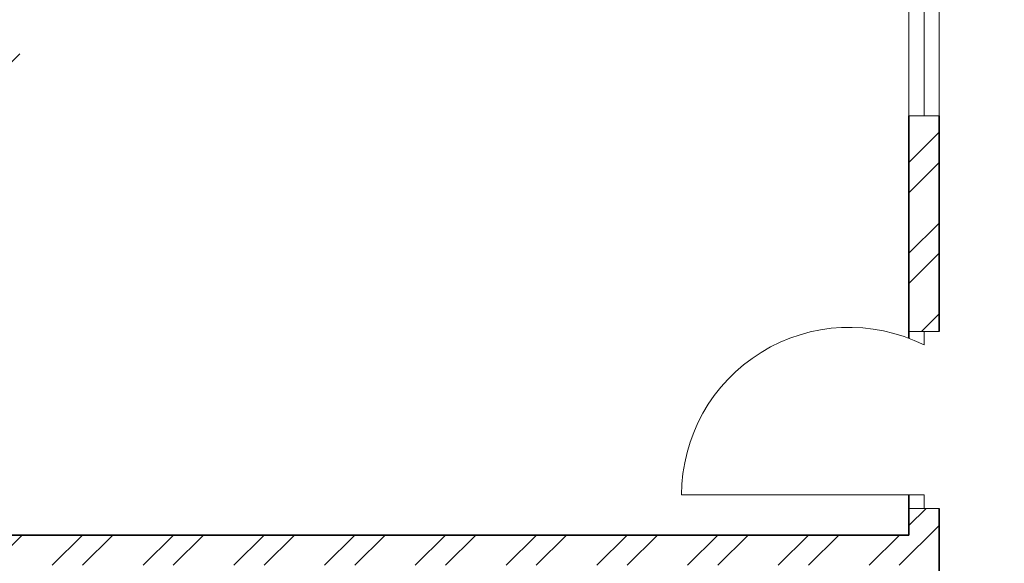
# Model space of a CAD drawing. Units: inches. Extents: x 1885 to 2748, y 783 to 2421.
# Tile 50 of 117: x 2311 to 2457, y 1683 to 1764. Entities that reach past the tile are written whole.
import ezdxf

# ---------------------------------------------------------------- set-up
doc = ezdxf.new("R2010")
doc.units = ezdxf.units.IN
for name, color, linetype, lineweight in [('A-DOOR', 31, 'Continuous', 18), ('A-GLAZ', 181, 'Continuous', 18), ('A-WALL', 7, 'Continuous', 35)]:
    doc.layers.add(name, color=color, linetype=linetype, lineweight=lineweight)
doc.layers.add('A-WALL-PATT', color=85, linetype='Continuous', lineweight=13, true_color=0x58ba48)

# ---------------------------------------------------------------- blocks, each defined once
blk = doc.blocks.new('WIN-60')
for p, q in [((0, 60), (4.5, 60)), ((0, 60), (0, 0)), ((4.5, 60), (2.25, 60)), ((2.25, 60), (2.25, 0)), ((4.5, 0), (4.5, 60)), ((2.25, 0), (0, 0)), ((0, 0), (4.5, 0))]:
    blk.add_line(p, q)

msp = doc.modelspace()

# ---------------------------------------------------------------- hatches: boundary and pattern name
at = {"layer": 'A-WALL-PATT'}
h = msp.add_hatch(dxfattribs=at)
h.set_pattern_fill('ANSI32', color=256)
h.paths.add_polyline_path([(2007.77, 2318.01), (1980.77, 2318.01), (1980.77, 2281.22), (1985.27, 2281.22), (1985.27, 2313.51), (2007.77, 2313.51), (2007.77, 2315.76)])
h.paths.add_polyline_path([(2094.32, 2318.01), (2067.77, 2318.01), (2067.77, 2313.51), (2094.32, 2313.51), (2094.32, 2315.76)])
h.paths.add_polyline_path([(2131.37, 2315.76), (2131.37, 2318.01), (2131.19, 2318.01), (2112.61, 2318.01), (2112.61, 2313.51), (2117.27, 2313.51), (2117.27, 2255.2), (2121.77, 2255.2), (2121.77, 2313.51), (2131.37, 2313.51)])
h.paths.add_polyline_path([(2190.51, 2318.01), (2155.37, 2318.01), (2155.37, 2313.51), (2169.77, 2313.51), (2169.77, 2229.51), (2121.77, 2229.51), (2121.77, 2233.45), (2119.52, 2233.45), (2117.27, 2233.45), (2117.27, 2201.1), (2121.77, 2201.1), (2121.77, 2225.01), (2169.77, 2225.01), (2169.77, 2165.01), (2306.27, 2165.01), (2306.27, 2066.01), (2310.77, 2066.01), (2344.27, 2066.01), (2486.27, 2066.01), (2486.27, 1886.01), (2483.02, 1886.01), (2483.02, 1881.51), (2486.27, 1881.51), (2486.27, 1880.68), (2490.77, 1880.68), (2490.77, 2070.51), (2344.27, 2070.51), (2310.77, 2070.51), (2310.77, 2165.01), (2310.77, 2173.64), (2308.52, 2173.64), (2306.27, 2173.64), (2306.27, 2169.51), (2174.27, 2169.51), (2174.27, 2313.51), (2190.51, 2313.51), (2190.51, 2315.76)])
h.paths.add_polyline_path([(1985.27, 2221.22), (1980.77, 2221.22), (1980.77, 2165.01), (1992.77, 2165.01), (1992.77, 2141.93), (1997.27, 2141.93), (1997.27, 2165.01), (2117.27, 2165.01), (2117.27, 2163.13), (2121.77, 2163.13), (2121.77, 2172.73), (2119.52, 2172.73), (2117.27, 2172.73), (2117.27, 2169.51), (1985.27, 2169.51)])
h.paths.add_polyline_path([(1997.27, 2105.93), (1992.77, 2105.93), (1992.77, 2070.51), (2016.77, 2070.51), (2016.77, 2059.12), (2019.02, 2059.12), (2021.27, 2059.12), (2021.27, 2070.51), (2117.27, 2070.51), (2117.27, 2022.51), (2114.42, 2022.51), (2114.42, 2018.01), (2123.63, 2018.01), (2123.63, 2020.26), (2123.63, 2022.51), (2121.77, 2022.51), (2121.77, 2142.59), (2119.52, 2142.59), (2117.27, 2142.59), (2117.27, 2075.01), (1997.27, 2075.01)])
h.paths.add_polyline_path([(2092.03, 2020.26), (2092.03, 2022.51), (2021.27, 2022.51), (2021.27, 2035.12), (2016.77, 2035.12), (2016.77, 2018.01), (2016.77, 1978.78), (2021.27, 1978.78), (2021.27, 2018.01), (2092.03, 2018.01)])
h.paths.add_polyline_path([(2260.94, 2022.51), (2153.1, 2022.51), (2153.1, 2020.26), (2153.1, 2018.01), (2155.27, 2018.01), (2155.27, 1886.01), (2107.63, 1886.01), (2107.63, 1881.51), (2182.91, 1881.51), (2182.91, 1883.76), (2182.91, 1886.01), (2159.77, 1886.01), (2159.77, 2018.01), (2260.94, 2018.01), (2260.94, 2020.26)])
h.paths.add_polyline_path([(2047.63, 1883.76), (2047.63, 1886.01), (2021.27, 1886.01), (2021.27, 1918.78), (2019.02, 1918.78), (2016.77, 1918.78), (2016.77, 1881.51), (2047.63, 1881.51)])
h.paths.add_polyline_path([(2306.36, 1883.76), (2306.36, 1886.01), (2296.27, 1886.01), (2296.27, 1982.01), (2316.54, 1982.01), (2316.54, 1984.26), (2316.54, 1986.51), (2296.27, 1986.51), (2296.27, 2022.51), (2289.28, 2022.51), (2289.28, 2018.01), (2291.77, 2018.01), (2291.77, 1886.01), (2242.91, 1886.01), (2242.91, 1881.51), (2306.36, 1881.51)], flags=17)
h.paths.add_polyline_path([(1985.27, 1843.01), (2021.6, 1843.01), (2021.53, 1845.44), (2021.48, 1847.51), (1980.77, 1847.51), (1980.77, 1809.45), (1985.27, 1809.45)])
h.paths.add_polyline_path([(2131.48, 1845.26), (2131.48, 1847.51), (2081.53, 1847.51), (2081.53, 1843.01), (2117.27, 1843.01), (2117.27, 1784.15), (2119.52, 1784.15), (2121.77, 1784.15), (2121.77, 1843.01), (2131.48, 1843.01)])
h.paths.add_polyline_path([(2203.89, 1847.51), (2155.48, 1847.51), (2155.48, 1843.01), (2169.77, 1843.01), (2169.77, 1759.01), (2121.77, 1759.01), (2121.77, 1761.46), (2117.27, 1761.46), (2117.27, 1730.43), (2121.77, 1730.43), (2121.77, 1754.51), (2177.42, 1754.51), (2177.42, 1756.76), (2177.42, 1759.01), (2174.27, 1759.01), (2174.27, 1843.01), (2203.89, 1843.01)])
h.paths.add_polyline_path([(2335.55, 1845.26), (2335.55, 1847.51), (2239.89, 1847.51), (2239.89, 1843.01), (2306.27, 1843.01), (2306.27, 1759.01), (2199.49, 1759.01), (2199.49, 1754.51), (2310.77, 1754.51), (2310.77, 1843.01), (2335.55, 1843.01)])
h.paths.add_polyline_path([(2348.77, 2022.51), (2344.27, 2022.51), (2344.27, 1986.51), (2341.68, 1986.51), (2341.68, 1982.01), (2344.27, 1982.01), (2344.27, 1886.01), (2330.36, 1886.01), (2330.36, 1881.51), (2361.63, 1881.51), (2361.63, 1883.76), (2361.63, 1886.01), (2348.77, 1886.01)], flags=17)
h.paths.add_polyline_path([(2283.25, 2315.76), (2283.25, 2318.01), (2238.51, 2318.01), (2238.51, 2313.51), (2283.25, 2313.51)], flags=17)
h.paths.add_polyline_path([(2363.27, 2348.01), (2388.68, 2348.01), (2388.68, 2350.26), (2388.68, 2352.51), (2358.77, 2352.51), (2358.77, 2348.01), (2358.77, 2318.01), (2344.48, 2318.01), (2344.48, 2313.51), (2358.77, 2313.51), (2358.77, 2229.51), (2310.77, 2229.51), (2310.77, 2231.95), (2306.27, 2231.95), (2306.27, 2205.61), (2310.77, 2205.61), (2310.77, 2225.01), (2358.77, 2225.01), (2358.77, 2211.51), (2452.33, 2211.51), (2452.33, 2213.76), (2452.33, 2216.01), (2363.27, 2216.01), (2363.27, 2318.01)])
h.paths.add_polyline_path([(2310.77, 2313.51), (2320.48, 2313.51), (2320.48, 2315.76), (2320.48, 2318.01), (2302.73, 2318.01), (2302.73, 2313.51), (2306.27, 2313.51), (2306.27, 2251.08), (2310.77, 2251.08)], flags=17)
h.paths.add_polyline_path([(2490.77, 2352.51), (2486.27, 2352.51), (2448.68, 2352.51), (2448.68, 2348.01), (2486.27, 2348.01), (2486.27, 2318.01), (2486.27, 2216.01), (2481.78, 2216.01), (2481.78, 2211.51), (2486.27, 2211.51), (2486.27, 2165.01), (2493.29, 2165.01), (2493.29, 2167.26), (2493.29, 2169.51), (2490.77, 2169.51), (2490.77, 2313.51), (2494.43, 2313.51), (2494.43, 2318.01), (2490.77, 2318.01)])
h.paths.add_polyline_path([(2534.65, 2318.01), (2515.69, 2318.01), (2515.69, 2313.51), (2534.65, 2313.51), (2534.65, 2315.76)])
h.paths.add_polyline_path([(2618.27, 2318.01), (2594.65, 2318.01), (2594.65, 2313.51), (2613.77, 2313.51), (2613.77, 2281.71), (2618.27, 2281.71)])
h.paths.add_polyline_path([(2618.27, 2221.71), (2613.77, 2221.71), (2613.77, 2169.51), (2554.02, 2169.51), (2554.02, 2165.01), (2613.77, 2165.01), (2613.77, 2152.88), (2618.27, 2152.88)])
h.paths.add_polyline_path([(2618.27, 2128.88), (2616.02, 2128.88), (2613.77, 2128.88), (2613.77, 2117.01), (2529.77, 2117.01), (2529.77, 2165.01), (2532.85, 2165.01), (2532.85, 2169.51), (2522.87, 2169.51), (2522.87, 2165.01), (2525.27, 2165.01), (2525.27, 2117.01), (2525.27, 2112.51), (2525.27, 2108.58), (2529.77, 2108.58), (2529.77, 2112.51), (2613.77, 2112.51), (2613.77, 2080.19), (2618.27, 2080.19)])
h.paths.add_polyline_path([(2618.27, 2044.19), (2616.02, 2044.19), (2613.77, 2044.19), (2613.77, 2015.51), (2529.77, 2015.51), (2529.77, 2088.58), (2527.52, 2088.58), (2525.27, 2088.58), (2525.27, 2011.01), (2613.77, 2011.01), (2613.77, 1956.75), (2618.27, 1956.75)])
h.paths.add_polyline_path([(2618.27, 1881.51), (2618.27, 1896.75), (2613.77, 1896.75), (2613.77, 1881.51), (2613.77, 1847.51), (2592.71, 1847.51), (2592.71, 1843.01), (2613.77, 1843.01), (2613.77, 1765.01), (2613.77, 1760.51), (2609.62, 1760.51), (2609.62, 1756.01), (2613.77, 1756.01), (2613.77, 1660.01), (2608.54, 1660.01), (2608.54, 1655.51), (2613.77, 1655.51), (2613.77, 1508.16), (2618.27, 1508.16)])
h.paths.add_polyline_path([(2565.77, 1843.01), (2569, 1843.01), (2569, 1847.51), (2490.77, 1847.51), (2490.77, 1849.7), (2488.52, 1849.7), (2486.27, 1849.7), (2486.27, 1847.51), (2477.27, 1847.51), (2477.27, 1838.51), (2477.27, 1821.49), (2486.27, 1821.49), (2486.27, 1838.51), (2561.27, 1838.51), (2561.27, 1765.01), (2486.27, 1765.01), (2486.27, 1786.16), (2477.27, 1786.16), (2477.27, 1765.01), (2477.27, 1756.01), (2486.27, 1756.01), (2565.77, 1756.01), (2585.62, 1756.01), (2585.62, 1758.26), (2585.62, 1760.51), (2565.77, 1760.51), (2565.77, 1765.01)])
h.paths.add_polyline_path([(2486.27, 1651.01), (2561.27, 1651.01), (2561.27, 1567.01), (2486.27, 1567.01), (2486.27, 1591.32), (2477.27, 1591.32), (2477.27, 1567.01), (2477.27, 1558.01), (2477.27, 1555.44), (2481.77, 1555.44), (2481.77, 1558.01), (2568.65, 1558.01), (2568.65, 1560.26), (2568.65, 1562.51), (2565.77, 1562.51), (2565.77, 1655.51), (2584.54, 1655.51), (2584.54, 1657.76), (2584.54, 1660.01), (2565.77, 1660.01), (2486.27, 1660.01), (2477.27, 1660.01), (2477.27, 1651.01), (2477.27, 1632.99), (2486.27, 1632.99)])
h.paths.add_polyline_path([(2449.97, 1883.76), (2449.97, 1886.01), (2421.63, 1886.01), (2421.63, 1881.51), (2449.97, 1881.51)], flags=17)
h.paths.add_polyline_path([(2447.27, 1847.51), (2395.55, 1847.51), (2395.55, 1843.01), (2442.77, 1843.01), (2442.77, 1809.27), (2447.27, 1809.27)])
h.paths.add_polyline_path([(1985.27, 1749.45), (1980.77, 1749.45), (1980.77, 1694.5), (1985.27, 1694.5), (1985.27, 1694.51), (1986.9, 1694.51), (1986.9, 1697.78), (1986.9, 1699.01), (1985.27, 1699.01)])
h.paths.add_polyline_path([(2152.77, 1699.01), (2121.77, 1699.01), (2121.77, 1703.67), (2119.52, 1703.67), (2117.27, 1703.67), (2117.27, 1699.01), (2009.22, 1699.01), (2009.22, 1694.51), (2148.27, 1694.51), (2148.27, 1692.63), (2152.77, 1692.63)])
h.paths.add_polyline_path([(2016.27, 1694.51), (2011.77, 1694.51), (2011.77, 1558.01), (2040.81, 1558.01), (2040.81, 1560.26), (2040.81, 1562.51), (2016.27, 1562.51)])
h.paths.add_polyline_path([(2152.77, 1663.02), (2150.52, 1663.02), (2148.27, 1663.02), (2148.27, 1562.51), (2100.81, 1562.51), (2100.81, 1558.01), (2165.12, 1558.01), (2165.12, 1560.26), (2165.12, 1562.51), (2152.77, 1562.51), (2152.77, 1610.51), (2224.77, 1610.51), (2224.77, 1607.99), (2229.27, 1607.99), (2229.27, 1615.01), (2152.77, 1615.01)])
h.paths.add_polyline_path([(2238.61, 1560.26), (2238.61, 1562.51), (2229.27, 1562.51), (2229.27, 1588.76), (2227.02, 1588.76), (2224.77, 1588.77), (2224.77, 1562.51), (2189.12, 1562.51), (2189.12, 1558.01), (2238.61, 1558.01)])
h.paths.add_polyline_path([(2336.02, 1560.26), (2336.02, 1562.51), (2310.77, 1562.51), (2310.77, 1656.35), (2308.52, 1656.35), (2306.27, 1656.35), (2306.27, 1562.51), (2286.61, 1562.51), (2286.61, 1558.01), (2336.02, 1558.01)])
h.paths.add_polyline_path([(2447.27, 1690.97), (2445.02, 1690.97), (2442.77, 1690.97), (2442.77, 1687.01), (2306.27, 1687.01), (2306.27, 1680.75), (2310.77, 1680.75), (2310.77, 1682.51), (2442.77, 1682.51), (2442.77, 1562.51), (2396.02, 1562.51), (2396.02, 1558.01), (2447.27, 1558.01)])
h.paths.add_polyline_path([(2447.27, 1749.27), (2445.02, 1749.27), (2442.77, 1749.27), (2442.77, 1717.23), (2447.27, 1717.23)])
h.paths.add_polyline_path([(2044.67, 1521.76), (2044.67, 1524.01), (2007.27, 1524.01), (2007.27, 1503.49), (2009.52, 1503.49), (2011.77, 1503.49), (2011.77, 1519.51), (2044.67, 1519.51)])
h.paths.add_polyline_path([(2177.97, 1521.76), (2177.97, 1524.01), (2104.67, 1524.01), (2104.67, 1519.51), (2145.77, 1519.51), (2145.77, 1387.51), (2143.37, 1387.51), (2143.37, 1383.01), (2251.59, 1383.01), (2251.59, 1385.26), (2251.59, 1387.51), (2150.27, 1387.51), (2150.27, 1519.51), (2177.97, 1519.51)])
h.paths.add_polyline_path([(2298.7, 1524.01), (2237.97, 1524.01), (2237.97, 1519.51), (2282.27, 1519.51), (2282.27, 1387.51), (2279.68, 1387.51), (2279.68, 1383.01), (2286.77, 1383.01), (2286.77, 1419.01), (2312.45, 1419.01), (2312.45, 1421.26), (2312.45, 1423.51), (2286.77, 1423.51), (2286.77, 1519.51), (2298.7, 1519.51), (2298.7, 1521.72)], flags=17)
h.paths.add_polyline_path([(2361.9, 1521.76), (2361.9, 1524.01), (2322.7, 1524.01), (2322.7, 1519.51), (2334.77, 1519.51), (2334.77, 1423.51), (2331.93, 1423.51), (2331.93, 1419.01), (2334.77, 1419.01), (2334.77, 1387.51), (2334.77, 1383.23), (2339.27, 1383.23), (2339.27, 1387.51), (2339.27, 1519.51), (2361.9, 1519.51)], flags=17)
h.paths.add_polyline_path([(2447.27, 1521.76), (2447.27, 1524.01), (2421.9, 1524.01), (2421.9, 1519.51), (2447.27, 1519.51)], flags=17)
h.paths.add_polyline_path([(2481.77, 1529.6), (2479.52, 1529.6), (2477.27, 1529.6), (2477.27, 1524.01), (2474.49, 1524.01), (2474.49, 1519.51), (2477.27, 1519.51), (2477.27, 1334.51), (2296.77, 1334.51), (2296.77, 1240.51), (2160.27, 1240.51), (2160.27, 1180.51), (2112.27, 1180.51), (2112.27, 1207.69), (2110.02, 1207.69), (2107.77, 1207.69), (2107.77, 1171.61), (2112.27, 1171.61), (2112.27, 1176.01), (2160.27, 1176.01), (2160.27, 1092.01), (2144.22, 1092.01), (2144.22, 1087.51), (2189.5, 1087.51), (2189.5, 1089.76), (2189.5, 1092.01), (2164.77, 1092.01), (2164.77, 1236.01), (2296.77, 1236.01), (2296.77, 1231.91), (2301.27, 1231.91), (2301.27, 1330.01), (2481.77, 1330.01), (2481.77, 1387.51)])
h.paths.add_polyline_path([(2618.27, 1448.16), (2613.77, 1448.16), (2613.77, 1382.51), (2529.77, 1382.51), (2525.27, 1382.51), (2525.27, 1307.06), (2529.77, 1307.06), (2529.77, 1378.01), (2613.77, 1378.01), (2613.77, 1354.99), (2618.27, 1354.99)])
h.paths.add_polyline_path([(2618.27, 1318.99), (2613.77, 1318.99), (2613.77, 1281.01), (2529.77, 1281.01), (2529.77, 1283.79), (2527.52, 1283.79), (2525.27, 1283.79), (2525.27, 1228.51), (2516.79, 1228.51), (2516.79, 1224.01), (2533.48, 1224.01), (2533.48, 1226.26), (2533.48, 1228.51), (2529.77, 1228.51), (2529.77, 1276.51), (2613.77, 1276.51), (2613.77, 1266.02), (2618.27, 1266.02)])
h.paths.add_polyline_path([(2618.27, 1134.96), (2613.77, 1134.96), (2613.77, 1092.01), (2594.54, 1092.01), (2594.54, 1087.51), (2618.27, 1087.51)])
h.paths.add_polyline_path([(2534.54, 1092.01), (2509.77, 1092.01), (2509.77, 1087.51), (2534.54, 1087.51), (2534.54, 1089.76)])
h.paths.add_polyline_path([(2481.27, 1224.01), (2484.12, 1224.01), (2484.12, 1226.26), (2484.12, 1228.51), (2476.77, 1228.51), (2476.77, 1198.51), (2471.61, 1198.51), (2471.61, 1194.01), (2476.77, 1194.01), (2476.77, 1062.01), (2436.89, 1062.01), (2436.89, 1057.51), (2476.77, 1057.51), (2481.27, 1057.51), (2481.27, 1062.01), (2481.27, 1087.51), (2485.35, 1087.51), (2485.35, 1089.76), (2485.35, 1092.01), (2481.27, 1092.01), (2481.27, 1117.51)])
h.paths.add_polyline_path([(2439.9, 1198.51), (2349.27, 1198.51), (2349.27, 1194.01), (2349.27, 1180.51), (2301.27, 1180.51), (2301.27, 1201.9), (2299.02, 1201.9), (2296.77, 1201.9), (2296.77, 1172.34), (2299.02, 1172.34), (2301.27, 1172.34), (2301.27, 1176.01), (2349.27, 1176.01), (2349.27, 1092.01), (2334.45, 1092.01), (2334.45, 1087.51), (2349.27, 1087.51), (2349.27, 1057.51), (2353.77, 1057.51), (2376.89, 1057.51), (2376.89, 1059.76), (2376.89, 1062.01), (2353.77, 1062.01), (2353.77, 1087.51), (2353.77, 1180.51), (2353.77, 1194.01), (2439.9, 1194.01), (2439.9, 1196.26)])
h.paths.add_polyline_path([(2270.6, 1089.76), (2270.6, 1092.01), (2249.5, 1092.01), (2249.5, 1087.51), (2270.6, 1087.51)], flags=17)
h.paths.add_polyline_path([(2310.45, 1092.01), (2301.27, 1092.01), (2301.27, 1153.29), (2296.77, 1153.29), (2296.77, 1092.01), (2293.79, 1092.01), (2293.79, 1087.51), (2310.45, 1087.51), (2310.45, 1089.76)], flags=17)
h.paths.add_polyline_path([(2112.27, 1150.33), (2110.02, 1150.33), (2107.77, 1150.33), (2107.77, 1092.01), (2104.47, 1092.01), (2104.47, 1087.51), (2120.22, 1087.51), (2120.22, 1089.76), (2120.22, 1092.01), (2112.27, 1092.01)])
h.paths.add_polyline_path([(2082.17, 1092.01), (2058.14, 1092.01), (2058.14, 1087.51), (2082.17, 1087.51), (2082.17, 1089.76)])
h.paths.add_polyline_path([(1975.77, 1145.64), (1971.27, 1145.64), (1971.27, 1087.51), (1980.77, 1087.51), (1998.14, 1087.51), (1998.14, 1089.76), (1998.14, 1092.01), (1985.27, 1092.01), (1975.77, 1092.01)])
h.paths.add_polyline_path([(2112.27, 1244.38), (2110.02, 1244.38), (2107.77, 1244.38), (2107.77, 1240.51), (1992.27, 1240.51), (1992.27, 1271.01), (1987.77, 1271.01), (1987.77, 1240.51), (1980.77, 1240.51), (1975.77, 1240.51), (1971.27, 1240.51), (1971.27, 1205.64), (1975.77, 1205.64), (1975.77, 1236.01), (2107.77, 1236.01), (2107.77, 1233.44), (2112.27, 1233.44), (2112.27, 1236.01)])
h.paths.add_polyline_path([(2112.27, 1383.01), (2114.78, 1383.01), (2114.78, 1385.26), (2114.78, 1387.51), (2102.48, 1387.51), (2102.48, 1383.01), (2107.77, 1383.01), (2107.77, 1335.01), (2011.77, 1335.01), (2011.77, 1349.94), (2007.27, 1349.94), (2007.27, 1335.01), (1987.77, 1335.01), (1987.77, 1330.51), (1987.77, 1307.01), (1992.27, 1307.01), (1992.27, 1330.51), (2007.27, 1330.51), (2107.77, 1330.51), (2107.77, 1264.71), (2112.27, 1264.71)])
h.paths.add_polyline_path([(2077.86, 1387.51), (2011.77, 1387.51), (2011.77, 1390.04), (2009.52, 1390.04), (2007.27, 1390.04), (2007.27, 1373.94), (2011.77, 1373.94), (2011.77, 1383.01), (2077.86, 1383.01)])
h.paths.add_polyline_path([(2011.77, 1443.49), (2007.27, 1443.49), (2007.27, 1410.25), (2011.77, 1410.25)])

# ---------------------------------------------------------------- linework, layer by layer
at = {"layer": 'A-DOOR'}
for p, q in [((2442.77, 1717.23), (2447.27, 1717.23)), ((2447.27, 1717.23), (2445.02, 1717.23)), ((2445.02, 1717.23), (2445.02, 1715.23)), ((2445.02, 1692.97), (2409.02, 1692.97)), ((2445.02, 1690.97), (2445.02, 1692.97)), ((2442.77, 1690.97), (2447.27, 1690.97)), ((2447.27, 1690.97), (2445.02, 1690.97))]:
    msp.add_line(p, q, dxfattribs=at)
msp.add_arc((2433.91, 1692.97), 24.88, 63.4692, 180, dxfattribs=at)
at = {"layer": 'A-WALL'}
for p, q in [((2442.77, 1749.27), (2442.77, 1716.22)), ((2447.27, 1749.27), (2447.27, 1717.23)), ((2442.77, 1692.97), (2442.77, 1687.01)), ((2447.27, 1690.97), (2447.27, 1558.01)), ((2306.27, 1687.01), (2442.77, 1687.01))]:
    msp.add_line(p, q, dxfattribs=at)

# ---------------------------------------------------------------- block references
at = {"layer": 'A-GLAZ', "extrusion": (0, 0, -1), "zscale": -1, "rotation": 180}
msp.add_blockref('WIN-60', (-2442.77, 1809.27), dxfattribs=at)

doc.saveas('drawing.dxf')
